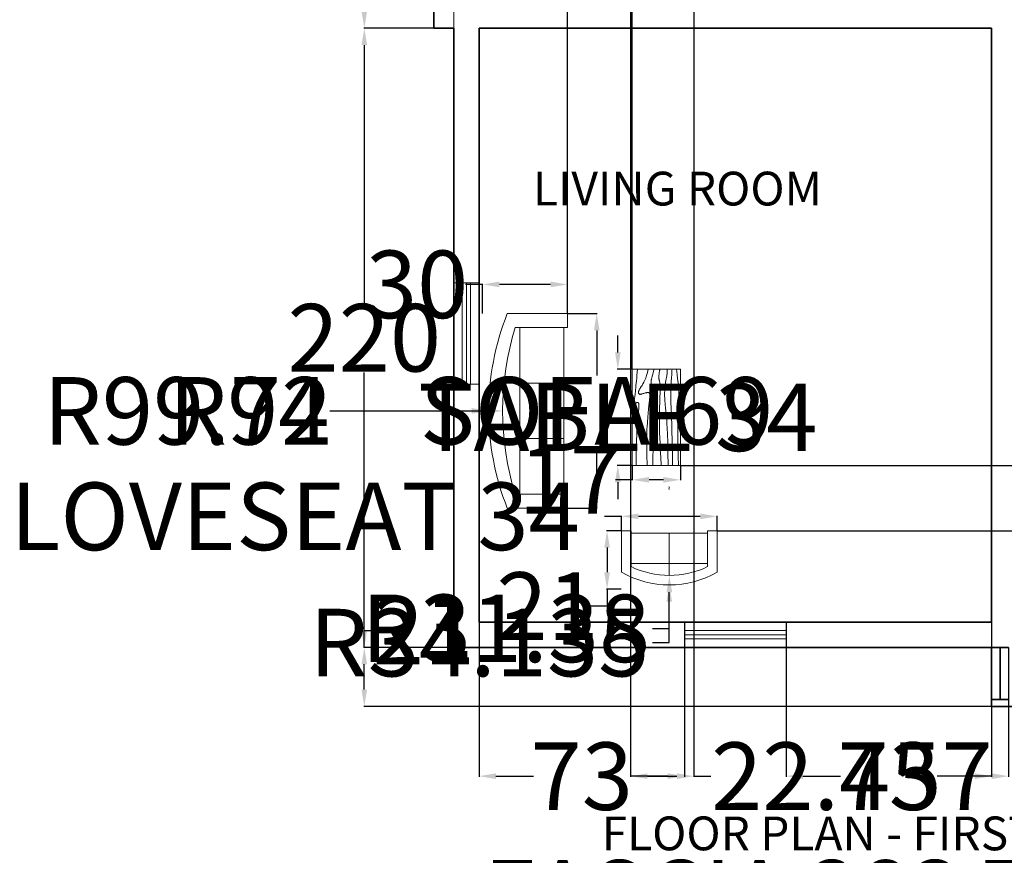
# Model space of a CAD drawing. Units: inches. Extents: x -15 to 1815, y 1023 to 2303.
# Tile 2 of 8: x 173 to 522, y 1772 to 2069. Entities that reach past the tile are written whole.
import ezdxf

# ---------------------------------------------------------------- set-up
doc = ezdxf.new("R2010")
doc.units = ezdxf.units.IN
doc.header["$MEASUREMENT"] = 0
for name, color, linetype, lineweight in [('A-ANNO-DIMS', 2, 'Continuous', 18), ('A-ANNO-TEXT', 7, 'Continuous', 25), ('A-AREA-IDEN', 7, 'Continuous', 18), ('A-FURN', 8, 'Continuous', 18), ('A-GLAZ', 4, 'Continuous', 18), ('A-REFR', 8, 'Continuous', 13), ('A-WALL', 7, 'Continuous', 35)]:
    doc.layers.add(name, color=color, linetype=linetype, lineweight=lineweight)
doc.styles.get("Standard").update_dxf_attribs({"font": 'arial.ttf'})
doc.dimstyles.get("Standard").update_dxf_attribs({"dimtxt": 24, "dimasz": 6, "dimexe": 0.18, "dimexo": 0.0625, "dimgap": 0.09, "dimtad": 0, "dimtih": 1, "dimtoh": 1, "dimdec": 0, "dimzin": 0, "dimdsep": 46, "dimlunit": 3, "dimtxsty": 'Standard', "dimcen": 0.09, "dimadec": 0, "dimazin": 0, "dimtfac": 1, "dimtdec": 0, "dimtofl": 0, "dimtmove": 0, "dimatfit": 3, "dimfxl": 1, "dimtolj": 1, "dimtzin": 0, "dimarcsym": 0})

# ---------------------------------------------------------------- blocks, each defined once
blk = doc.blocks.new('Sofa - Roundback Loveseat 5 ft.')
for p, q in [((0, -32.44198), (0, -5.99998)), ((-24, -33.99998), (-24, -11.46958)), ((24.00004, -33.99998), (24.00004, -11.46958)), ((-23.9998, -13.38178), (23.99986, -13.38178)), ((-24, -32.44198), (24.00004, -32.44198))]:
    blk.add_line(p, q)
for points in [[(-24, -33.99998), (-30, -33.99998), (-30, -7.99998)], [(30.00004, -7.99998), (30.00004, -33.99998), (24.00004, -33.99998)]]:
    blk.add_lwpolyline(points)
for centre, radius, start, end in [((0, -60.24998), 60.24998, 60.13715, 119.8628), ((0, -61.38438), 55.38444, 64.32083, 115.6792)]:
    blk.add_arc(centre, radius, start, end)
blk = doc.blocks.new('Sofa - Roundback 7 ft.')
for p, q in [((-12.00002, -32.4421), (-12.00003, -6.5971)), ((11.99997, -32.4421), (11.99998, -6.5971)), ((-36.000027, -34), (-36.000027, -11.4696)), ((35.99998, -34), (35.99998, -11.4696)), ((-35.999844, -13.3819), (35.9998, -13.3819)), ((-36.000027, -32.4421), (35.99998, -32.4421))]:
    blk.add_line(p, q)
for points in [[(-36.000027, -34), (-42.000027, -34), (-42.000027, -8)], [(41.99998, -8), (41.99998, -34), (35.99998, -34)]]:
    blk.add_lwpolyline(points)
for centre, radius, start, end in [((0, -114.25), 114.25, 68.43141, 111.5686), ((-0.00001, -127.1968), 121.1968, 72.72033, 107.2797)]:
    blk.add_arc(centre, radius, start, end)
blk = doc.blocks.new('Table - Rectangular Woodgrain 60 x 30 in.')
for p, q in [((0, 0), (0, -30)), ((60, 0), (0, 0)), ((60, -30), (60, 0)), ((0, -30), (60, -30))]:
    blk.add_line(p, q)
for points in [[(0, -2.4), (4.8155, -2.418), (9.0302, -2.4688), (12.709, -2.5477), (15.9167, -2.65), (18.7181, -2.7711), (21.1781, -2.9063), (23.3616, -3.0508), (25.3333, -3.2), (27.1477, -3.3495), (28.8172, -3.4958), (30.3437, -3.636), (31.7291, -3.7667), (32.9756, -3.8849), (34.0849, -3.9875), (35.059, -4.0714), (35.9, -4.1334), (36.6114, -4.1711), (37.2041, -4.1854), (37.6906, -4.1779), (38.0833, -4.15), (38.3948, -4.1034), (38.6375, -4.0396), (38.8239, -3.9602), (38.9666, -3.8667), (39.0764, -3.7608), (39.1573, -3.6448), (39.2116, -3.521), (39.2416, -3.3917), (39.2498, -3.2593), (39.2385, -3.1261), (39.21, -2.9944), (39.1666, -2.8667), (39.111, -2.7447), (39.0468, -2.6281), (38.978, -2.5163), (38.9083, -2.4083), (38.8418, -2.3035), (38.7823, -2.201), (38.7337, -2.1001), (38.7, -2), (38.6844, -1.9003), (38.6875, -1.8021), (38.7094, -1.707), (38.75, -1.6167), (38.8094, -1.5326), (38.8875, -1.4563), (38.9844, -1.3893), (39.1, -1.3333), (39.2351, -1.2896), (39.3937, -1.2583), (39.5804, -1.2396), (39.8, -1.2333), (40.057, -1.2396), (40.3562, -1.2583), (40.7023, -1.2896), (41.1, -1.3333), (41.5547, -1.3895), (42.0755, -1.4573), (42.6721, -1.5361), (43.3542, -1.625), (44.1316, -1.7233), (45.014, -1.8302), (46.0114, -1.9449), (47.1333, -2.0667), (48.3862, -2.1947), (49.7625, -2.3281), (51.2513, -2.4663), (52.8416, -2.6083), (54.5226, -2.7535), (56.2833, -2.9011), (58.1127, -3.0501), (60, -3.2)], [(0, -9.2), (6.5759, -9.0858), (11.9385, -9.0365), (16.2527, -9.0418), (19.6833, -9.0917), (22.3952, -9.1759), (24.5531, -9.2844), (26.322, -9.4069), (27.8666, -9.5333), (29.3241, -9.6553), (30.7203, -9.7719), (32.0532, -9.8837), (33.3208, -9.9917), (34.5213, -10.0965), (35.6526, -10.199), (36.7128, -10.2999), (37.7, -10.4), (38.6129, -10.4996), (39.4531, -10.5969), (40.223, -10.6895), (40.925, -10.775), (41.5613, -10.8512), (42.1344, -10.9156), (42.6465, -10.966), (43.1, -11), (43.4976, -11.0158), (43.8437, -11.0136), (44.143, -10.9942), (44.4, -10.9583), (44.6195, -10.9069), (44.8062, -10.8406), (44.9648, -10.7603), (45.1, -10.6667), (45.2155, -10.5598), (45.3114, -10.4365), (45.3871, -10.2929), (45.4416, -10.125), (45.4743, -9.929), (45.4844, -9.7011), (45.4709, -9.4371), (45.4333, -9.1333), (45.3716, -8.7883), (45.2896, -8.4104), (45.1919, -8.0107), (45.0833, -7.6), (44.9685, -7.1893), (44.8521, -6.7896), (44.7388, -6.4117), (44.6333, -6.0667), (44.54, -5.7628), (44.4614, -5.4979), (44.4001, -5.2675), (44.3583, -5.0667), (44.3384, -4.8909), (44.3427, -4.7354), (44.3736, -4.5956), (44.4333, -4.4667), (44.5236, -4.3453), (44.6427, -4.2333), (44.7884, -4.1339), (44.9583, -4.05), (45.1501, -3.9849), (45.3614, -3.9417), (45.59, -3.9234), (45.8333, -3.9333), (46.0915, -3.9749), (46.3734, -4.0531), (46.6906, -4.1736), (47.0542, -4.3417), (47.4756, -4.5629), (47.9661, -4.8427), (48.5372, -5.1866), (49.2, -5.6), (49.9676, -6.0844), (50.8594, -6.625), (51.8965, -7.2031), (53.1, -7.8), (54.491, -8.3969), (56.0906, -8.975), (57.9199, -9.5156), (60, -10)], [(0, -12.8), (5.1847, -12.9322), (9.6213, -13.0323), (13.3963, -13.1059), (16.5958, -13.1583), (19.3063, -13.1952), (21.614, -13.2219), (23.6054, -13.2439), (25.3666, -13.2667), (26.9728, -13.2947), (28.4531, -13.3281), (29.8256, -13.3663), (31.1083, -13.4083), (32.3191, -13.4535), (33.476, -13.501), (34.597, -13.5501), (35.7, -13.6), (36.7984, -13.6497), (37.8875, -13.6979), (38.9578, -13.743), (40, -13.7833), (41.0047, -13.8174), (41.9625, -13.8438), (42.864, -13.8607), (43.7, -13.8667), (44.4631, -13.8604), (45.1552, -13.8417), (45.7801, -13.8104), (46.3416, -13.7667), (46.8439, -13.7104), (47.2906, -13.6417), (47.6858, -13.5604), (48.0333, -13.4667), (48.3375, -13.3608), (48.6042, -13.2448), (48.8396, -13.121), (49.05, -12.9917), (49.2417, -12.8593), (49.4208, -12.7261), (49.5937, -12.5944), (49.7667, -12.4667), (49.9452, -12.3451), (50.1323, -12.2313), (50.3303, -12.1268), (50.5416, -12.0333), (50.7686, -11.9524), (51.0135, -11.8854), (51.2788, -11.8341), (51.5666, -11.8), (51.8785, -11.7843), (52.2116, -11.7865), (52.562, -11.8059), (52.926, -11.8417), (53.2998, -11.8931), (53.6795, -11.9594), (54.0614, -12.0397), (54.4416, -12.1333), (54.8223, -12.2401), (55.2293, -12.3625), (55.6942, -12.5037), (56.2489, -12.6667), (56.9251, -12.8547), (57.7545, -13.0708), (58.7689, -13.3182), (60, -13.6)], [(0, -18), (5.124, -17.7273), (9.6609, -17.5057), (13.6705, -17.3303), (17.2125, -17.1958), (20.3467, -17.0973), (23.1328, -17.0297), (25.6307, -16.9878), (27.9, -16.9667), (29.9928, -16.9617), (31.9302, -16.9703), (33.7254, -16.9907), (35.3917, -17.0208), (36.9423, -17.0588), (38.3906, -17.1026), (39.7499, -17.1503), (41.0333, -17.2), (42.2519, -17.2496), (43.4073, -17.2969), (44.4986, -17.3395), (45.525, -17.375), (46.4858, -17.4012), (47.3802, -17.4156), (48.2074, -17.416), (48.9667, -17.4), (49.6583, -17.3662), (50.2872, -17.3167), (50.8595, -17.2547), (51.3812, -17.1833), (51.8584, -17.1057), (52.2971, -17.025), (52.7034, -16.9443), (53.0833, -16.8667), (53.443, -16.7951), (53.789, -16.7313), (54.128, -16.6768), (54.4666, -16.6334), (54.8115, -16.6024), (55.1693, -16.5854), (55.5465, -16.5841), (55.95, -16.6), (56.3828, -16.6337), (56.8346, -16.6823), (57.2915, -16.7418), (57.7396, -16.8084), (58.165, -16.878), (58.5539, -16.9469), (58.8924, -17.0111), (59.1666, -17.0667), (59.3679, -17.1107), (59.5078, -17.1438), (59.6032, -17.1675), (59.6708, -17.1833), (59.7275, -17.193), (59.7901, -17.1979), (59.8753, -17.1998), (60, -17.2)], [(0, -22.4), (8.0098, -22.2501), (14.4094, -22.1011), (19.4168, -21.9535), (23.25, -21.8083), (26.1269, -21.6663), (28.2656, -21.5281), (29.884, -21.3947), (31.2, -21.2667), (32.3967, -21.1448), (33.5172, -21.0292), (34.5697, -20.9198), (35.5625, -20.8167), (36.5037, -20.7198), (37.4015, -20.6292), (38.2642, -20.5448), (39.1, -20.4667), (39.9164, -20.3951), (40.7187, -20.3313), (41.5117, -20.2768), (42.3, -20.2333), (43.0883, -20.2024), (43.8812, -20.1854), (44.6836, -20.1841), (45.5, -20.2), (46.3328, -20.234), (47.1747, -20.2844), (48.0163, -20.3488), (48.8479, -20.425), (49.66, -20.5106), (50.4429, -20.6031), (51.1872, -20.7004), (51.8833, -20.8), (52.5246, -20.8999), (53.1166, -20.9995), (53.6681, -21.0983), (54.1875, -21.1958), (54.6834, -21.2919), (55.1646, -21.3859), (55.6394, -21.4777), (56.1167, -21.5667), (56.6028, -21.6515), (57.0961, -21.7266), (57.5929, -21.7852), (58.0896, -21.8208), (58.5823, -21.8268), (59.0674, -21.7964), (59.5412, -21.723), (60, -21.6)], [(0, -25.2), (8.6355, -25.0504), (15.7026, -24.9031), (21.4049, -24.7606), (25.9458, -24.625), (29.529, -24.4988), (32.3578, -24.3844), (34.6359, -24.284), (36.5667, -24.2), (38.3213, -24.1341), (39.9417, -24.0854), (41.437, -24.0523), (42.8167, -24.0333), (44.0901, -24.0268), (45.2667, -24.0313), (46.3557, -24.0451), (47.3667, -24.0667), (48.309, -24.0947), (49.1928, -24.1287), (50.0284, -24.168), (50.826, -24.2125), (51.5959, -24.2617), (52.3483, -24.3151), (53.0935, -24.3725), (53.8417, -24.4334), (54.6009, -24.497), (55.3699, -24.561), (56.1454, -24.6226), (56.9239, -24.6792), (57.7021, -24.7279), (58.4764, -24.7662), (59.2435, -24.7911), (60, -24.8)], [(0, -28.8), (5.6867, -28.6681), (10.45, -28.5698), (14.407, -28.5012), (17.675, -28.4584), (20.3711, -28.4374), (22.6125, -28.4344), (24.5164, -28.4455), (26.2, -28.4667), (27.762, -28.4947), (29.2276, -28.5281), (30.6033, -28.5663), (31.8958, -28.6084), (33.1118, -28.6535), (34.2578, -28.7011), (35.3405, -28.7501), (36.3666, -28.8), (37.3443, -28.8497), (38.288, -28.8974), (39.2137, -28.9412), (40.1375, -28.9792), (41.0753, -29.0093), (42.0432, -29.0297), (43.0572, -29.0384), (44.1333, -29.0333), (45.2936, -29.0114), (46.5843, -28.9641), (48.0579, -28.8816), (49.7666, -28.7542), (51.7629, -28.5721), (54.0989, -28.3255), (56.8272, -28.0048), (60, -27.6)]]:
    blk.add_lwpolyline(points)
blk = doc.blocks.new('Window - Wood Frame 36 in. Wide plan')
for p, q in [((0, 7.5), (0, -1.5)), ((36, 7.5), (36, -1.5)), ((0, 4.5), (36, 4.5)), ((0, 3), (36, 3)), ((0, 1.5), (36, 1.5))]:
    blk.add_line(p, q)
blk = doc.blocks.new('*D27')
at = {"layer": 'A-ANNO-DIMS', "color": 0, "lineweight": -2, "transparency": 16777216}
for p, q in [((386.4, 1892.89), (380.4, 1892.89)), ((386.4, 1887.85), (386.4, 1893.07)), ((414.39, 1892.89), (392.4, 1892.89)), ((420.39, 1887.85), (420.39, 1893.07))]:
    blk.add_line(p, q, dxfattribs=at)
at = {"layer": 'A-ANNO-DIMS', "color": 0, "transparency": 16777216}
for points in [[(392.4, 1893.89), (392.4, 1891.89), (386.4, 1892.89)], [(414.39, 1893.89), (414.39, 1891.89), (420.39, 1892.89)]]:
    blk.add_solid(points, dxfattribs=at)
at = {"layer": 'Defpoints', "color": 0, "transparency": 16777216}
for p in [(386.4, 1892.89), (386.4, 1887.79), (420.39, 1887.79)]:
    blk.add_point(p, dxfattribs=at)
at = {"layer": 'A-ANNO-DIMS', "color": 0, "transparency": 16777216, "insert": (270.53, 1892.89), "char_height": 24, "attachment_point": 5}
blk.add_mtext('\\A1;LOVESEAT 34', dxfattribs=at)
blk = doc.blocks.new('*D28')
at = {"layer": 'A-ANNO-DIMS', "color": 0, "lineweight": -2, "transparency": 16777216}
for p, q in [((386.34, 1887.79), (381.12, 1887.79)), ((381.3, 1881.79), (381.3, 1873.02)), ((386.34, 1867.02), (381.12, 1867.02)), ((381.3, 1867.02), (381.3, 1861.02)), ((381.3, 1861.02), (375.3, 1861.02))]:
    blk.add_line(p, q, dxfattribs=at)
at = {"layer": 'A-ANNO-DIMS', "color": 0, "transparency": 16777216}
for points in [[(380.3, 1881.79), (382.3, 1881.79), (381.3, 1887.79)], [(380.3, 1873.02), (382.3, 1873.02), (381.3, 1867.02)]]:
    blk.add_solid(points, dxfattribs=at)
at = {"layer": 'Defpoints', "color": 0, "transparency": 16777216}
for p in [(386.4, 1887.79), (381.3, 1867.02), (386.4, 1867.02)]:
    blk.add_point(p, dxfattribs=at)
at = {"layer": 'A-ANNO-DIMS', "color": 0, "transparency": 16777216, "insert": (360.13, 1861.02), "char_height": 24, "attachment_point": 5}
blk.add_mtext('\\A1;21', dxfattribs=at)
blk = doc.blocks.new('*D29')
at = {"layer": 'A-ANNO-DIMS', "color": 0, "lineweight": -2, "transparency": 16777216}
for p, q in [((367.31, 1964.92), (377.79, 1964.92)), ((377.61, 1958.92), (377.61, 1942.87)), ((377.61, 1901.81), (377.61, 1917.86)), ((367.31, 1895.81), (377.79, 1895.81))]:
    blk.add_line(p, q, dxfattribs=at)
at = {"layer": 'A-ANNO-DIMS', "color": 0, "transparency": 16777216}
for points in [[(376.61, 1958.92), (378.61, 1958.92), (377.61, 1964.92)], [(376.61, 1901.81), (378.61, 1901.81), (377.61, 1895.81)]]:
    blk.add_solid(points, dxfattribs=at)
at = {"layer": 'Defpoints', "color": 0, "transparency": 16777216}
for p in [(367.25, 1964.92), (377.61, 1964.92), (367.25, 1895.81)]:
    blk.add_point(p, dxfattribs=at)
at = {"layer": 'A-ANNO-DIMS', "color": 0, "transparency": 16777216, "insert": (377.61, 1930.36), "char_height": 24, "attachment_point": 5}
blk.add_mtext('\\A1;SOFA 69', dxfattribs=at)
blk = doc.blocks.new('*D30')
at = {"layer": 'A-ANNO-DIMS', "color": 0, "lineweight": -2, "transparency": 16777216}
for p, q in [((337.08, 1975.29), (331.08, 1975.29)), ((337.08, 1964.98), (337.08, 1975.47)), ((361.25, 1975.29), (343.08, 1975.29)), ((367.25, 1964.98), (367.25, 1975.47))]:
    blk.add_line(p, q, dxfattribs=at)
at = {"layer": 'A-ANNO-DIMS', "color": 0, "transparency": 16777216}
for points in [[(343.08, 1976.29), (343.08, 1974.29), (337.08, 1975.29)], [(361.25, 1976.29), (361.25, 1974.29), (367.25, 1975.29)]]:
    blk.add_solid(points, dxfattribs=at)
at = {"layer": 'Defpoints', "color": 0, "transparency": 16777216}
for p in [(337.08, 1975.29), (337.08, 1964.92), (367.25, 1964.92)]:
    blk.add_point(p, dxfattribs=at)
at = {"layer": 'A-ANNO-DIMS', "color": 0, "transparency": 16777216, "insert": (313.85, 1975.29), "char_height": 24, "attachment_point": 5}
blk.add_mtext('\\A1;30', dxfattribs=at)
blk = doc.blocks.new('*D31')
at = {"layer": 'A-ANNO-DIMS', "color": 0, "lineweight": -2, "transparency": 16777216}
for p, q in [((385.12, 1951.14), (385.12, 1957.14)), ((390.18, 1945.14), (384.94, 1945.14)), ((390.18, 1910.99), (384.94, 1910.99)), ((385.12, 1904.99), (385.12, 1898.99))]:
    blk.add_line(p, q, dxfattribs=at)
at = {"layer": 'A-ANNO-DIMS', "color": 0, "transparency": 16777216}
for points in [[(384.12, 1951.14), (386.12, 1951.14), (385.12, 1945.14)], [(384.12, 1904.99), (386.12, 1904.99), (385.12, 1910.99)]]:
    blk.add_solid(points, dxfattribs=at)
at = {"layer": 'Defpoints', "color": 0, "transparency": 16777216}
for p in [(385.12, 1945.14), (390.24, 1945.14), (390.24, 1910.99)]:
    blk.add_point(p, dxfattribs=at)
at = {"layer": 'A-ANNO-DIMS', "color": 0, "transparency": 16777216, "insert": (385.12, 1928.07), "char_height": 24, "attachment_point": 5}
blk.add_mtext('\\A1;TABLE 34', dxfattribs=at)
blk = doc.blocks.new('*D32')
at = {"layer": 'A-ANNO-DIMS', "color": 0, "lineweight": -2, "transparency": 16777216}
for p, q in [((390.24, 1910.93), (390.24, 1905.69)), ((407.31, 1910.93), (407.31, 1905.69)), ((390.24, 1905.87), (384.24, 1905.87)), ((401.31, 1905.87), (396.24, 1905.87))]:
    blk.add_line(p, q, dxfattribs=at)
at = {"layer": 'A-ANNO-DIMS', "color": 0, "transparency": 16777216}
for points in [[(396.24, 1906.87), (396.24, 1904.87), (390.24, 1905.87)], [(401.31, 1906.87), (401.31, 1904.87), (407.31, 1905.87)]]:
    blk.add_solid(points, dxfattribs=at)
at = {"layer": 'Defpoints', "color": 0, "transparency": 16777216}
for p in [(390.24, 1910.99), (407.31, 1910.99), (390.24, 1905.87)]:
    blk.add_point(p, dxfattribs=at)
at = {"layer": 'A-ANNO-DIMS', "color": 0, "transparency": 16777216, "insert": (368.09, 1905.87), "char_height": 24, "attachment_point": 5}
blk.add_mtext('\\A1;17', dxfattribs=at)
blk = doc.blocks.new('*D33')
at = {"layer": 'A-ANNO-DIMS', "color": 0, "lineweight": -2, "transparency": 16777216}
for p, q in [((393.59, 2104.63), (393.59, 2096.83)), ((444.77, 2104.63), (444.77, 2096.83)), ((399.59, 2097.01), (438.77, 2097.01)), ((444.77, 2097.01), (450.77, 2097.01))]:
    blk.add_line(p, q, dxfattribs=at)
at = {"layer": 'A-ANNO-DIMS', "color": 0, "transparency": 16777216}
for points in [[(399.59, 2098.01), (399.59, 2096.01), (393.59, 2097.01)], [(438.77, 2098.01), (438.77, 2096.01), (444.77, 2097.01)]]:
    blk.add_solid(points, dxfattribs=at)
at = {"layer": 'Defpoints', "color": 0, "transparency": 16777216}
for p in [(393.59, 2104.69), (444.77, 2104.69), (444.77, 2097.01)]:
    blk.add_point(p, dxfattribs=at)
at = {"layer": 'A-ANNO-DIMS', "color": 0, "transparency": 16777216, "insert": (565.73, 2097.01), "char_height": 24, "attachment_point": 5}
blk.add_mtext('\\A1;DINING SET 51', dxfattribs=at)
blk = doc.blocks.new('*D57')
at = {"layer": 'A-ANNO-DIMS', "color": 0, "lineweight": -2, "transparency": 16777216}
for p, q in [((317.89, 1716.39), (317.89, 1758.98)), ((323.89, 1758.8), (327.1, 1758.8)), ((595.01, 1758.8), (591.8, 1758.8)), ((601.01, 1716.39), (601.01, 1758.98))]:
    blk.add_line(p, q, dxfattribs=at)
at = {"layer": 'A-ANNO-DIMS', "color": 0, "transparency": 16777216}
for points in [[(323.89, 1759.8), (323.89, 1757.8), (317.89, 1758.8)], [(595.01, 1759.8), (595.01, 1757.8), (601.01, 1758.8)]]:
    blk.add_solid(points, dxfattribs=at)
at = {"layer": 'Defpoints', "color": 0, "transparency": 16777216}
for p in [(601.01, 1758.8), (317.89, 1716.33), (601.01, 1716.33)]:
    blk.add_point(p, dxfattribs=at)
at = {"layer": 'A-ANNO-DIMS', "color": 0, "transparency": 16777216, "insert": (459.45, 1758.8), "char_height": 24, "attachment_point": 5}
blk.add_mtext('\\A1;FASCIA 283 TYP.', dxfattribs=at)
blk = doc.blocks.new('*D61')
at = {"layer": 'A-ANNO-DIMS', "color": 0, "lineweight": -2, "transparency": 16777216}
for p, q in [((295.1, 1846.33), (295.1, 1852.33)), ((295.1, 1852.33), (301.1, 1852.33)), ((326.77, 1846.33), (294.92, 1846.33)), ((295.1, 1831.33), (295.1, 1840.33)), ((517.77, 1825.33), (294.92, 1825.33))]:
    blk.add_line(p, q, dxfattribs=at)
at = {"layer": 'A-ANNO-DIMS', "color": 0, "transparency": 16777216}
for points in [[(294.1, 1840.33), (296.1, 1840.33), (295.1, 1846.33)], [(294.1, 1831.33), (296.1, 1831.33), (295.1, 1825.33)]]:
    blk.add_solid(points, dxfattribs=at)
at = {"layer": 'Defpoints', "color": 0, "transparency": 16777216}
for p in [(295.1, 1846.33), (326.83, 1846.33), (517.83, 1825.33)]:
    blk.add_point(p, dxfattribs=at)
at = {"layer": 'A-ANNO-DIMS', "color": 0, "transparency": 16777216, "insert": (316.27, 1852.33), "char_height": 24, "attachment_point": 5}
blk.add_mtext('\\A1;21', dxfattribs=at)
blk = doc.blocks.new('*D62')
at = {"layer": 'A-ANNO-DIMS', "color": 0, "lineweight": -2, "transparency": 16777216}
for p, q in [((319.77, 2066.33), (294.92, 2066.33)), ((295.1, 2060.33), (295.1, 1968.67)), ((295.1, 1852.33), (295.1, 1943.98)), ((326.77, 1846.33), (294.92, 1846.33))]:
    blk.add_line(p, q, dxfattribs=at)
at = {"layer": 'A-ANNO-DIMS', "color": 0, "transparency": 16777216}
for points in [[(294.1, 2060.33), (296.1, 2060.33), (295.1, 2066.33)], [(294.1, 1852.33), (296.1, 1852.33), (295.1, 1846.33)]]:
    blk.add_solid(points, dxfattribs=at)
at = {"layer": 'Defpoints', "color": 0, "transparency": 16777216}
for p in [(295.1, 2066.33), (319.83, 2066.33), (326.83, 1846.33)]:
    blk.add_point(p, dxfattribs=at)
at = {"layer": 'A-ANNO-DIMS', "color": 0, "transparency": 16777216, "insert": (295.1, 1956.33), "char_height": 24, "attachment_point": 5}
blk.add_mtext('\\A1;220', dxfattribs=at)
blk = doc.blocks.new('*D63')
at = {"layer": 'A-ANNO-DIMS', "color": 0, "lineweight": -2, "transparency": 16777216}
for p, q in [((319.77, 2258.33), (294.92, 2258.33)), ((295.1, 2252.33), (295.1, 2174.67)), ((295.1, 2072.33), (295.1, 2149.98)), ((319.77, 2066.33), (294.92, 2066.33))]:
    blk.add_line(p, q, dxfattribs=at)
at = {"layer": 'A-ANNO-DIMS', "color": 0, "transparency": 16777216}
for points in [[(294.1, 2252.33), (296.1, 2252.33), (295.1, 2258.33)], [(294.1, 2072.33), (296.1, 2072.33), (295.1, 2066.33)]]:
    blk.add_solid(points, dxfattribs=at)
at = {"layer": 'Defpoints', "color": 0, "transparency": 16777216}
for p in [(295.1, 2258.33), (319.83, 2258.33), (319.83, 2066.33)]:
    blk.add_point(p, dxfattribs=at)
at = {"layer": 'A-ANNO-DIMS', "color": 0, "transparency": 16777216, "insert": (295.1, 2162.33), "char_height": 24, "attachment_point": 5}
blk.add_mtext('\\A1;192', dxfattribs=at)
blk = doc.blocks.new('*D64')
at = {"layer": 'A-ANNO-DIMS', "color": 0, "lineweight": -2, "transparency": 16777216}
for p, q in [((523.834675, 1846.264776), (523.834675, 1800.414776)), ((569.834675, 1846.264776), (569.834675, 1800.414776)), ((517.834675, 1800.594776), (511.834675, 1800.594776)), ((575.834675, 1800.594776), (581.834675, 1800.594776))]:
    blk.add_line(p, q, dxfattribs=at)
at = {"layer": 'A-ANNO-DIMS', "color": 0, "transparency": 16777216}
for points in [[(517.834675, 1801.594776), (517.834675, 1799.594776), (523.834675, 1800.594776)], [(575.834675, 1801.594776), (575.834675, 1799.594776), (569.834675, 1800.594776)]]:
    blk.add_solid(points, dxfattribs=at)
at = {"layer": 'Defpoints', "color": 0, "transparency": 16777216}
for p in [(523.834675, 1846.327276), (569.834675, 1846.327276), (569.834675, 1800.594776)]:
    blk.add_point(p, dxfattribs=at)
at = {"layer": 'A-ANNO-DIMS', "color": 0, "transparency": 16777216, "insert": (546.834675, 1800.594776), "char_height": 24, "attachment_point": 5}
blk.add_mtext('\\A1;46', dxfattribs=at)
blk = doc.blocks.new('*D66')
at = {"layer": 'A-ANNO-DIMS', "color": 0, "lineweight": -2, "transparency": 16777216}
for p, q in [((335.83, 1855.26), (335.83, 1800.41)), ((408.83, 1855.26), (408.83, 1800.41)), ((341.83, 1800.59), (355.15, 1800.59)), ((402.83, 1800.59), (389.52, 1800.59))]:
    blk.add_line(p, q, dxfattribs=at)
at = {"layer": 'A-ANNO-DIMS', "color": 0, "transparency": 16777216}
for points in [[(341.83, 1801.59), (341.83, 1799.59), (335.83, 1800.59)], [(402.83, 1801.59), (402.83, 1799.59), (408.83, 1800.59)]]:
    blk.add_solid(points, dxfattribs=at)
at = {"layer": 'Defpoints', "color": 0, "transparency": 16777216}
for p in [(335.83, 1855.33), (408.83, 1855.33), (408.83, 1800.59)]:
    blk.add_point(p, dxfattribs=at)
at = {"layer": 'A-ANNO-DIMS', "color": 0, "transparency": 16777216, "insert": (372.33, 1800.59), "char_height": 24, "attachment_point": 5}
blk.add_mtext('\\A1;73', dxfattribs=at)
blk = doc.blocks.new('*D67')
at = {"layer": 'A-ANNO-DIMS', "color": 0, "lineweight": -2, "transparency": 16777216}
for p, q in [((444.83, 1855.26), (444.83, 1800.41)), ((517.83, 1855.26), (517.83, 1800.41)), ((450.83, 1800.59), (464.15, 1800.59)), ((511.83, 1800.59), (498.52, 1800.59))]:
    blk.add_line(p, q, dxfattribs=at)
at = {"layer": 'A-ANNO-DIMS', "color": 0, "transparency": 16777216}
for points in [[(450.83, 1801.59), (450.83, 1799.59), (444.83, 1800.59)], [(511.83, 1801.59), (511.83, 1799.59), (517.83, 1800.59)]]:
    blk.add_solid(points, dxfattribs=at)
at = {"layer": 'Defpoints', "color": 0, "transparency": 16777216}
for p in [(444.83, 1855.33), (517.83, 1855.33), (517.83, 1800.59)]:
    blk.add_point(p, dxfattribs=at)
at = {"layer": 'A-ANNO-DIMS', "color": 0, "transparency": 16777216, "insert": (481.33, 1800.59), "char_height": 24, "attachment_point": 5}
blk.add_mtext('\\A1;73', dxfattribs=at)
blk = doc.blocks.new('*D68')
at = {"layer": 'A-ANNO-DIMS', "color": 0, "lineweight": -2, "transparency": 16777216}
for p, q in [((367.25, 1964.98), (367.25, 2283.24)), ((373.25, 2283.06), (384.24, 2283.06)), ((390.24, 1945.2), (390.24, 2283.24)), ((390.24, 2283.06), (396.24, 2283.06))]:
    blk.add_line(p, q, dxfattribs=at)
at = {"layer": 'A-ANNO-DIMS', "color": 0, "transparency": 16777216}
for points in [[(373.25, 2284.06), (373.25, 2282.06), (367.25, 2283.06)], [(384.24, 2284.06), (384.24, 2282.06), (390.24, 2283.06)]]:
    blk.add_solid(points, dxfattribs=at)
at = {"layer": 'Defpoints', "color": 0, "transparency": 16777216}
for p in [(390.24, 2283.06), (367.25, 1964.92), (390.24, 1945.14)]:
    blk.add_point(p, dxfattribs=at)
at = {"layer": 'A-ANNO-DIMS', "color": 0, "transparency": 16777216, "insert": (446.3, 2283.06), "char_height": 24, "attachment_point": 5}
blk.add_mtext('\\A1;22.994', dxfattribs=at)
blk = doc.blocks.new('*D69')
at = {"layer": 'A-ANNO-DIMS', "color": 0, "lineweight": -2, "transparency": 16777216}
for p, q in [((407.38, 1910.99), (751.75, 1910.99)), ((751.57, 1904.99), (751.57, 1893.79)), ((420.46, 1887.79), (751.75, 1887.79)), ((751.57, 1887.79), (751.57, 1881.79)), ((751.57, 1881.79), (745.57, 1881.79))]:
    blk.add_line(p, q, dxfattribs=at)
at = {"layer": 'A-ANNO-DIMS', "color": 0, "transparency": 16777216}
for points in [[(750.57, 1904.99), (752.57, 1904.99), (751.57, 1910.99)], [(750.57, 1893.79), (752.57, 1893.79), (751.57, 1887.79)]]:
    blk.add_solid(points, dxfattribs=at)
at = {"layer": 'Defpoints', "color": 0, "transparency": 16777216}
for p in [(407.31, 1910.99), (420.39, 1887.79), (751.57, 1887.79)]:
    blk.add_point(p, dxfattribs=at)
at = {"layer": 'A-ANNO-DIMS', "color": 0, "transparency": 16777216, "insert": (695.46, 1881.79), "char_height": 24, "attachment_point": 5}
blk.add_mtext('\\A1;23.203', dxfattribs=at)
blk = doc.blocks.new('*D78')
at = {"layer": 'A-ANNO-DIMS', "color": 0, "lineweight": -2, "transparency": 16777216}
for p, q in [((389.65, 2155.45), (389.65, 1800.41)), ((412.11, 2155.45), (412.11, 1800.41)), ((395.65, 1800.59), (406.11, 1800.59)), ((412.11, 1800.59), (418.11, 1800.59))]:
    blk.add_line(p, q, dxfattribs=at)
at = {"layer": 'A-ANNO-DIMS', "color": 0, "transparency": 16777216}
for points in [[(395.65, 1801.59), (395.65, 1799.59), (389.65, 1800.59)], [(406.11, 1801.59), (406.11, 1799.59), (412.11, 1800.59)]]:
    blk.add_solid(points, dxfattribs=at)
at = {"layer": 'Defpoints', "color": 0, "transparency": 16777216}
for p in [(389.65, 2155.51), (412.11, 2155.51), (412.11, 1800.59)]:
    blk.add_point(p, dxfattribs=at)
at = {"layer": 'A-ANNO-DIMS', "color": 0, "transparency": 16777216, "insert": (468.22, 1800.59), "char_height": 24, "attachment_point": 5}
blk.add_mtext('\\A1;22.457', dxfattribs=at)
blk = doc.blocks.new('*D124')
at = {"layer": 'A-ANNO-DIMS', "color": 0, "lineweight": -2, "transparency": 16777216}
for p, q in [((284.38, 1930.36), (338.21, 1930.36)), ((443.83, 1930.36), (444.01, 1930.36)), ((443.92, 1930.27), (443.92, 1930.45))]:
    blk.add_line(p, q, dxfattribs=at)
at = {"layer": 'A-ANNO-DIMS', "color": 0, "transparency": 16777216}
blk.add_solid([(338.21, 1931.36), (338.21, 1929.36), (344.21, 1930.36)], dxfattribs=at)
at = {"layer": 'Defpoints', "color": 0, "transparency": 16777216}
for p in [(344.21, 1930.36), (443.92, 1930.36)]:
    blk.add_point(p, dxfattribs=at)
at = {"layer": 'A-ANNO-DIMS', "color": 0, "transparency": 16777216, "insert": (232.43, 1930.36), "char_height": 24, "attachment_point": 5}
blk.add_mtext('\\A1;R99.72', dxfattribs=at)
blk = doc.blocks.new('*D125')
at = {"layer": 'A-ANNO-DIMS', "color": 0, "lineweight": -2, "transparency": 16777216}
for p, q in [((282.87, 1930.36), (333.27, 1930.36)), ((433.18, 1930.36), (433.36, 1930.36)), ((433.27, 1930.27), (433.27, 1930.45))]:
    blk.add_line(p, q, dxfattribs=at)
at = {"layer": 'A-ANNO-DIMS', "color": 0, "transparency": 16777216}
blk.add_solid([(333.27, 1931.36), (333.27, 1929.36), (339.27, 1930.36)], dxfattribs=at)
at = {"layer": 'Defpoints', "color": 0, "transparency": 16777216}
for p in [(339.27, 1930.36), (433.27, 1930.36)]:
    blk.add_point(p, dxfattribs=at)
at = {"layer": 'A-ANNO-DIMS', "color": 0, "transparency": 16777216, "insert": (254.16, 1930.36), "char_height": 24, "attachment_point": 5}
blk.add_mtext('\\A1;R94', dxfattribs=at)
blk = doc.blocks.new('*D126')
at = {"layer": 'A-ANNO-DIMS', "color": 0, "lineweight": -2, "transparency": 16777216}
for p, q in [((403.31, 1902.66), (403.49, 1902.66)), ((403.4, 1902.57), (403.4, 1902.75)), ((403.4, 1848.05), (403.4, 1862.53)), ((397.4, 1848.05), (403.4, 1848.05))]:
    blk.add_line(p, q, dxfattribs=at)
at = {"layer": 'A-ANNO-DIMS', "color": 0, "transparency": 16777216}
blk.add_solid([(402.4, 1862.53), (404.4, 1862.53), (403.4, 1868.53)], dxfattribs=at)
at = {"layer": 'Defpoints', "color": 0, "transparency": 16777216}
for p in [(403.4, 1902.66), (403.4, 1868.53)]:
    blk.add_point(p, dxfattribs=at)
at = {"layer": 'A-ANNO-DIMS', "color": 0, "transparency": 16777216, "insert": (335.92, 1848.05), "char_height": 24, "attachment_point": 5}
blk.add_mtext('\\A1;R34.135', dxfattribs=at)
blk = doc.blocks.new('*D127')
at = {"layer": 'A-ANNO-DIMS', "color": 0, "lineweight": -2, "transparency": 16777216}
for p, q in [((403.31, 1903.31), (403.49, 1903.31)), ((403.4, 1903.22), (403.4, 1903.4)), ((403.4, 1853.1), (403.4, 1865.93)), ((397.4, 1853.1), (403.4, 1853.1))]:
    blk.add_line(p, q, dxfattribs=at)
at = {"layer": 'A-ANNO-DIMS', "color": 0, "transparency": 16777216}
blk.add_solid([(402.4, 1865.93), (404.4, 1865.93), (403.4, 1871.93)], dxfattribs=at)
at = {"layer": 'Defpoints', "color": 0, "transparency": 16777216}
for p in [(403.4, 1903.31), (403.4, 1871.93)]:
    blk.add_point(p, dxfattribs=at)
at = {"layer": 'A-ANNO-DIMS', "color": 0, "transparency": 16777216, "insert": (345.3, 1853.1), "char_height": 24, "attachment_point": 5}
blk.add_mtext('\\A1;R31.38', dxfattribs=at)

msp = doc.modelspace()

# ---------------------------------------------------------------- linework, layer by layer
at = {"layer": 'A-REFR'}
msp.add_ray((326.8347, 1846.3273), (0, 1), dxfattribs=at)
at = {"layer": 'A-WALL'}
for p, q in [((319.8347, 2258.3273), (319.8347, 2066.3273)), ((319.8347, 2066.3273), (326.8347, 2066.3273)), ((326.8347, 2066.3273), (326.8347, 1846.3273)), ((517.8347, 2066.3273), (335.8347, 2066.3273)), ((335.8347, 2066.3273), (335.8347, 2060.3273)), ((517.8347, 2066.3273), (517.8347, 1855.3273)), ((335.8347, 2060.3273), (335.8347, 1855.3273)), ((335.8347, 1855.3273), (517.8347, 1855.3273)), ((326.8347, 1846.3273), (523.8347, 1846.3273)), ((517.8347, 1846.3273), (517.8347, 1825.3273)), ((520.8347, 1846.3273), (520.8347, 1827.7829)), ((523.8347, 1827.7829), (517.8347, 1827.7829)), ((575.8347, 1825.3273), (517.8347, 1825.3273))]:
    msp.add_line(p, q, dxfattribs=at)

# ---------------------------------------------------------------- block references
at = {"layer": 'A-FURN'}
for name, p, xscale, yscale, zscale, rotation in [('Sofa - Roundback 7 ft.', (339.2723, 1930.3637), 0.8227604582614757, 0.8227604582614757, 0.8227604582614757, 90), ('Table - Rectangular Woodgrain 60 x 30 in.', (390.2404, 1910.9946), 0.5691123726662638, 0.5691123726662638, 0.5691123726662638, 90), ('Sofa - Roundback Loveseat 5 ft.', (403.397, 1868.5284), 0.5665553462166426, 0.5665553462166426, 0.5665553462166426, 180)]:
    msp.add_blockref(name, p, dxfattribs=dict(at, xscale=xscale, yscale=yscale, zscale=zscale, rotation=rotation))
at = {"layer": 'A-GLAZ'}
for p, rotation in [((334.3347, 1939.8273), 90.00000000000006), ((444.8347, 1853.8273), 180)]:
    msp.add_blockref('Window - Wood Frame 36 in. Wide plan', p, dxfattribs=dict(at, rotation=rotation))

# ---------------------------------------------------------------- texts
at = {"layer": 'A-ANNO-TEXT'}
msp.add_text('FLOOR PLAN - FIRST FLOOR', height=12, dxfattribs=at).set_placement((379.3855, 1774.2654))
at = {"layer": 'A-AREA-IDEN'}
msp.add_text('LIVING ROOM', height=12, dxfattribs=at).set_placement((354.9455, 2003.3191))

# ---------------------------------------------------------------- dimensions: what is measured, and where the dimension line sits
at = {"layer": 'A-ANNO-DIMS'}
for base, p1, p2, override, picture, middle in [((390.2404, 2283.0598), (367.2461, 1964.9196), (390.2404, 1945.1413), {"dimdec": 3, "dimlfac": 1, "dimrnd": 0, "dimzin": 0, "dimdsep": 46, "dimlunit": 2}, '*D68', (446.3031, 2283.0598)), ((412.1112, 1800.5948), (389.6546, 2155.5101), (412.1112, 2155.5101), {"dimdec": 3, "dimlfac": 1, "dimrnd": 0, "dimzin": 0, "dimdsep": 46, "dimlunit": 2}, '*D78', (468.223, 1800.5948)), ((408.8347, 1800.5948), (335.8347, 1855.3273), (408.8347, 1855.3273), {"dimdec": 0, "dimlfac": 1, "dimrnd": 0, "dimzin": 0, "dimdsep": 46, "dimlunit": 2}, '*D66', (372.3347, 1800.5948)), ((517.8347, 1800.5948), (444.8347, 1855.3273), (517.8347, 1855.3273), {"dimdec": 0, "dimlfac": 1, "dimrnd": 0, "dimzin": 0, "dimdsep": 46, "dimlunit": 2}, '*D67', (481.3347, 1800.5948)), ((569.8347, 1800.5948), (523.8347, 1846.3273), (569.8347, 1846.3273), {"dimdec": 0, "dimlfac": 1, "dimrnd": 0, "dimzin": 0, "dimdsep": 46, "dimlunit": 2}, '*D64', (546.8347, 1800.5948))]:
    dim = msp.add_linear_dim(base=base, p1=p1, p2=p2, dimstyle='Standard', override=override, dxfattribs=at)
    dim.commit()
    dim.dimension.update_dxf_attribs({"geometry": picture, "text_midpoint": middle})
for base, p1, p2, angle, override, picture, middle in [((295.1022, 2258.3273), (319.8347, 2066.3273), (319.8347, 2258.3273), 90, {"dimdec": 0, "dimlfac": 1, "dimrnd": 0, "dimzin": 0, "dimdsep": 46, "dimlunit": 2}, '*D63', (295.1022, 2162.3273)), ((295.1022, 2066.3273), (326.8347, 1846.3273), (319.8347, 2066.3273), 90, {"dimdec": 0, "dimlfac": 1, "dimrnd": 0, "dimzin": 0, "dimdsep": 46, "dimlunit": 2}, '*D62', (295.1022, 1956.3273)), ((337.0782, 1975.2864), (367.2461, 1964.9196), (337.0782, 1964.9196), 180, {"dimdec": 0, "dimlfac": 1, "dimrnd": 0, "dimzin": 0, "dimdsep": 46, "dimlunit": 2}, '*D30', (313.8477, 1975.2864)), ((390.2404, 1905.8725), (407.3138, 1910.9946), (390.2404, 1910.9946), 180, {"dimdec": 0, "dimlfac": 1, "dimrnd": 0, "dimzin": 0, "dimdsep": 46, "dimlunit": 2}, '*D32', (368.0904, 1905.8725)), ((751.5672, 1887.7913), (407.3138, 1910.9946), (420.3937, 1887.7913), 90, {"dimdec": 3, "dimlfac": 1, "dimrnd": 0, "dimzin": 0, "dimdsep": 46, "dimlunit": 2}, '*D69', (695.4553, 1881.7913)), ((381.3013, 1867.0176), (386.4003, 1887.7913), (386.4003, 1867.0176), 270, {"dimdec": 0, "dimlfac": 1, "dimrnd": 0, "dimzin": 0, "dimdsep": 46, "dimlunit": 2}, '*D28', (360.1336, 1861.0176)), ((295.1022, 1846.3273), (517.8347, 1825.3273), (326.8347, 1846.3273), 90, {"dimdec": 0, "dimlfac": 1, "dimrnd": 0, "dimzin": 0, "dimdsep": 46, "dimlunit": 2}, '*D61', (316.2699, 1852.3273))]:
    dim = msp.add_linear_dim(base=base, p1=p1, p2=p2, angle=angle, dimstyle='Standard', override=override, dxfattribs=at)
    dim.commit()
    dim.dimension.update_dxf_attribs({"geometry": picture, "text_midpoint": middle})
for base, p1, p2, text, picture, middle in [((444.7686, 2097.011), (393.5857, 2104.6884), (444.7686, 2104.6884), 'DINING SET <>', '*D33', (565.7263, 2097.011)), ((601.0103, 1758.7967), (317.8894, 1716.3286), (601.0103, 1716.3286), 'FASCIA <> TYP.', '*D57', (459.4498, 1758.7967))]:
    dim = msp.add_linear_dim(base=base, p1=p1, p2=p2, text=text, dimstyle='Standard', override={"dimdec": 0, "dimlfac": 1, "dimrnd": 0, "dimzin": 0, "dimdsep": 46, "dimlunit": 2}, dxfattribs=at)
    dim.commit()
    dim.dimension.update_dxf_attribs({"geometry": picture, "text_midpoint": middle})
for base, p1, p2, angle, text, picture, middle in [((377.6129, 1964.9196), (367.2461, 1895.8077), (367.2461, 1964.9196), 90, 'SOFA <>', '*D29', (377.6129, 1930.3636)), ((385.1184, 1945.1413), (390.2404, 1910.9946), (390.2404, 1945.1413), 90, 'TABLE <>', '*D31', (385.1184, 1928.0679)), ((386.4003, 1892.8903), (420.3937, 1887.7913), (386.4003, 1887.7913), 180, 'LOVESEAT <>', '*D27', (270.5341, 1892.8903))]:
    dim = msp.add_linear_dim(base=base, p1=p1, p2=p2, angle=angle, text=text, dimstyle='Standard', override={"dimdec": 0, "dimlfac": 1, "dimrnd": 0, "dimzin": 0, "dimdsep": 46, "dimlunit": 2}, dxfattribs=at)
    dim.commit()
    dim.dimension.update_dxf_attribs({"geometry": picture, "text_midpoint": middle})
for center, mpoint, override, picture, middle in [((443.9248, 1930.3636), (344.2088, 1930.364), {"dimdec": 2, "dimlfac": 1, "dimrnd": 0, "dimzin": 0, "dimdsep": 46, "dimlunit": 2}, '*D124', (284.3793, 1930.3642)), ((433.2726, 1930.3637), (339.2723, 1930.364), {"dimdec": 0, "dimlfac": 1, "dimrnd": 0, "dimzin": 0, "dimdsep": 46, "dimlunit": 2}, '*D125', (282.872, 1930.3642)), ((403.397, 1902.6634), (403.397, 1868.5284), {"dimdec": 3, "dimlfac": 1, "dimrnd": 0, "dimzin": 0, "dimdsep": 46, "dimlunit": 2}, '*D126', (335.9155, 1848.0474)), ((403.397, 1903.3061), (403.397, 1871.9277), {"dimdec": 2, "dimlfac": 1, "dimrnd": 0, "dimzin": 0, "dimdsep": 46, "dimlunit": 2}, '*D127', (345.3043, 1853.1007))]:
    dim = msp.add_radius_dim(center=center, mpoint=mpoint, dimstyle='Standard', override=override, dxfattribs=at)
    dim.commit()
    dim.dimension.update_dxf_attribs({"geometry": picture, "text_midpoint": middle, "dimtype": 164})

doc.saveas('drawing.dxf')
